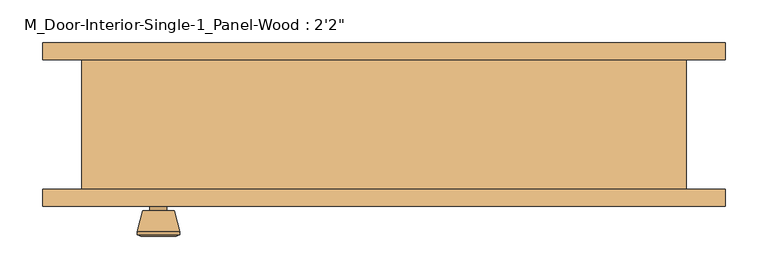
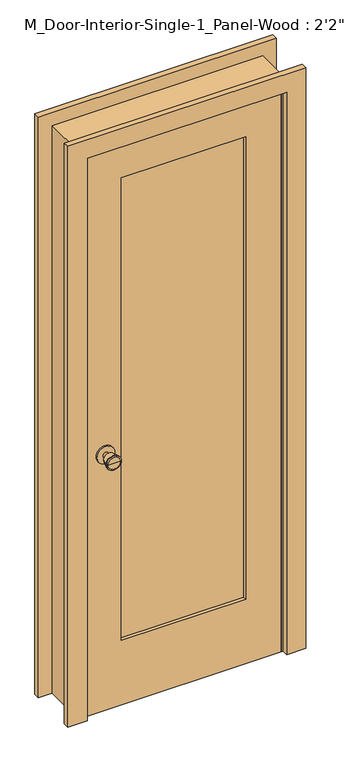
"""IFC4 building model written with IfcOpenShell, lengths in millimetres: door geometry."""

from ifc_helpers import new_model, si_unit, point, frame, frame_2d, origin, place, context, project, spatial, polyline, circle_curve, trimmed, segment, composite_curve, outline, extrude, faceted_brep, source, transform, mapped, element, save
from ifc_brep_helpers import plane_surface, cylinder_surface, revolved_surface, advanced_brep


def door_acb0f330(model_context):
    return source(origin(), model_context, "Body", "SolidModel", [
        advanced_brep(
        [(-265.2, -32.025, 914.4), (-275.2, -32.025, 914.4), (-255.2, -32.025, 914.4), (-244.7241324, 16.975, 914.4), (-285.6758676, 16.975, 914.4), (-265.2, 16.975, 914.4), (-240.2, 15.1471319, 914.4), (-290.2, 15.1471319, 914.4), (-240.2, 11.6834537, 914.4), (-290.2, 11.6834537, 914.4), (-246.563764, -13.025, 914.4), (-283.836236, -13.025, 914.4), (-255.2, -13.025, 914.4), (-275.2, -13.025, 914.4)],
        [
            (0, 1),
            (1, 2, circle_curve(frame((-265.2, -32.025, 914.4), z_axis=(0.0, -1.0, 0.0), x_axis=(-1.0, 0.0, 0.0)), 10.0)),
            (2, 0),
            (2, 1, circle_curve(frame((-265.2, -32.025, 914.4), z_axis=(0.0, -1.0, 0.0), x_axis=(-1.0, 0.0, 0.0)), 10.0)),
            (3, 4, circle_curve(frame((-265.2, 16.975, 914.4), z_axis=(0.0, 1.0, 0.0), x_axis=(-1.0, 0.0, 0.0)), 20.4758676)),
            (4, 5),
            (5, 3),
            (4, 3, circle_curve(frame((-265.2, 16.975, 914.4), z_axis=(0.0, 1.0, 0.0), x_axis=(-1.0, 0.0, 0.0)), 20.4758676)),
            (6, 7, circle_curve(frame((-265.2, 15.1471319, 914.4), z_axis=(0.0, 1.0, 0.0), x_axis=(-1.0, 0.0, 0.0)), 25.0)),
            (7, 4),
            (3, 6),
            (7, 6, circle_curve(frame((-265.2, 15.1471319, 914.4), z_axis=(0.0, 1.0, 0.0), x_axis=(-1.0, 0.0, 0.0)), 25.0)),
            (8, 9, circle_curve(frame((-265.2, 11.6834537, 914.4), z_axis=(0.0, 1.0, 0.0), x_axis=(-1.0, 0.0, 0.0)), 25.0)),
            (9, 7),
            (6, 8),
            (9, 8, circle_curve(frame((-265.2, 11.6834537, 914.4), z_axis=(0.0, 1.0, 0.0), x_axis=(-1.0, 0.0, 0.0)), 25.0)),
            (10, 11, circle_curve(frame((-265.2, -13.025, 914.4), z_axis=(0.0, 1.0, 0.0), x_axis=(-1.0, 0.0, 0.0)), 18.636236)),
            (11, 9),
            (8, 10),
            (11, 10, circle_curve(frame((-265.2, -13.025, 914.4), z_axis=(0.0, 1.0, 0.0), x_axis=(-1.0, 0.0, 0.0)), 18.636236)),
            (12, 13, circle_curve(frame((-265.2, -13.025, 914.4), z_axis=(0.0, 1.0, 0.0), x_axis=(-1.0, 0.0, 0.0)), 10.0)),
            (13, 11),
            (10, 12),
            (13, 12, circle_curve(frame((-265.2, -13.025, 914.4), z_axis=(0.0, 1.0, 0.0), x_axis=(-1.0, 0.0, 0.0)), 10.0)),
            (1, 13),
            (12, 2),
        ],
        [
            plane_surface(frame((-265.2, -32.025, 914.4), z_axis=(0.0, -1.0, 0.0), x_axis=(-1.0, 0.0, 0.0))),
            plane_surface(frame((-265.2, 16.975, 914.4), z_axis=(0.0, 1.0, 0.0), x_axis=(-1.0, 0.0, 0.0))),
            revolved_surface(polyline([(-285.6758676, 16.975, 914.4), (-290.2, 15.1471319, 914.4)]), (-265.2, -32.025, 914.4), (0.0, -1.0, 0.0)),
            cylinder_surface(frame((-265.2, -32.025, 914.4), z_axis=(0.0, -1.0, 0.0), x_axis=(-1.0, 0.0, 0.0)), 25.0),
            revolved_surface(polyline([(-290.2, 11.6834537, 914.4), (-283.836236, -13.025, 914.4)]), (-265.2, -32.025, 914.4), (0.0, -1.0, 0.0)),
            plane_surface(frame((-265.2, -13.025, 914.4), z_axis=(0.0, -1.0, 0.0), x_axis=(-1.0, 0.0, 0.0))),
            cylinder_surface(frame((-265.2, -32.025, 914.4), z_axis=(0.0, -1.0, 0.0), x_axis=(-1.0, 0.0, 0.0)), 10.0),
        ],
        [
            (0, [[1, 2, 3]]),
            (0, [[-3, 4, -1]]),
            (1, [[5, 6, 7]]),
            (1, [[8, -7, -6]]),
            (2, [[9, 10, -5, 11]]),
            (2, [[12, -11, -8, -10]]),
            (3, [[13, 14, -9, 15]]),
            (3, [[16, -15, -12, -14]]),
            (4, [[17, 18, -13, 19]]),
            (4, [[20, -19, -16, -18]]),
            (5, [[21, 22, -17, 23]]),
            (5, [[24, -23, -20, -22]]),
            (6, [[-2, 25, -21, 26]]),
            (6, [[-4, -26, -24, -25]]),
        ],
    ),
        extrude(outline(composite_curve([segment(trimmed(circle_curve(frame_2d((914.4, -265.2)), 30.0), [point((914.4, -295.2))], [point((914.4, -235.2))], False, "CARTESIAN"), True, "CONTINUOUS"), segment(trimmed(circle_curve(frame_2d((914.4, -265.2)), 30.0), [point((914.4, -235.2))], [point((914.4, -295.2))], False, "CARTESIAN"), True, "CONTINUOUS")], self_intersect=False)), frame((0.0, -38.025, 0.0), z_axis=(0.0, 1.0, 0.0), x_axis=(0.0, 0.0, 1.0)), (0.0, 0.0, 1.0), 6.0),
        advanced_brep(
        [(-265.2, -79.025, 914.4), (-255.2, -79.025, 914.4), (-275.2, -79.025, 914.4), (-244.7241324, -128.025, 914.4), (-265.2, -128.025, 914.4), (-285.6758676, -128.025, 914.4), (-240.2, -126.1971319, 914.4), (-290.2, -126.1971319, 914.4), (-240.2, -122.7334537, 914.4), (-290.2, -122.7334537, 914.4), (-246.563764, -98.025, 914.4), (-283.836236, -98.025, 914.4), (-255.2, -98.025, 914.4), (-275.2, -98.025, 914.4)],
        [
            (0, 1),
            (1, 2, circle_curve(frame((-265.2, -79.025, 914.4), z_axis=(0.0, 1.0, 0.0), x_axis=(-1.0, 0.0, 0.0)), 10.0)),
            (2, 0),
            (2, 1, circle_curve(frame((-265.2, -79.025, 914.4), z_axis=(0.0, 1.0, 0.0), x_axis=(-1.0, 0.0, 0.0)), 10.0)),
            (3, 4),
            (4, 5),
            (5, 3, circle_curve(frame((-265.2, -128.025, 914.4), z_axis=(0.0, -1.0, 0.0), x_axis=(-1.0, 0.0, 0.0)), 20.4758676)),
            (3, 5, circle_curve(frame((-265.2, -128.025, 914.4), z_axis=(0.0, -1.0, 0.0), x_axis=(-1.0, 0.0, 0.0)), 20.4758676)),
            (6, 3),
            (5, 7),
            (7, 6, circle_curve(frame((-265.2, -126.1971319, 914.4), z_axis=(0.0, -1.0, 0.0), x_axis=(-1.0, 0.0, 0.0)), 25.0)),
            (6, 7, circle_curve(frame((-265.2, -126.1971319, 914.4), z_axis=(0.0, -1.0, 0.0), x_axis=(-1.0, 0.0, 0.0)), 25.0)),
            (8, 6),
            (7, 9),
            (9, 8, circle_curve(frame((-265.2, -122.7334537, 914.4), z_axis=(0.0, -1.0, 0.0), x_axis=(-1.0, 0.0, 0.0)), 25.0)),
            (8, 9, circle_curve(frame((-265.2, -122.7334537, 914.4), z_axis=(0.0, -1.0, 0.0), x_axis=(-1.0, 0.0, 0.0)), 25.0)),
            (10, 8),
            (9, 11),
            (11, 10, circle_curve(frame((-265.2, -98.025, 914.4), z_axis=(0.0, -1.0, 0.0), x_axis=(-1.0, 0.0, 0.0)), 18.636236)),
            (10, 11, circle_curve(frame((-265.2, -98.025, 914.4), z_axis=(0.0, -1.0, 0.0), x_axis=(-1.0, 0.0, 0.0)), 18.636236)),
            (12, 10),
            (11, 13),
            (13, 12, circle_curve(frame((-265.2, -98.025, 914.4), z_axis=(0.0, -1.0, 0.0), x_axis=(-1.0, 0.0, 0.0)), 10.0)),
            (12, 13, circle_curve(frame((-265.2, -98.025, 914.4), z_axis=(0.0, -1.0, 0.0), x_axis=(-1.0, 0.0, 0.0)), 10.0)),
            (1, 12),
            (13, 2),
        ],
        [
            plane_surface(frame((-265.2, -79.025, 914.4), z_axis=(0.0, 1.0, 0.0), x_axis=(-1.0, 0.0, 0.0))),
            plane_surface(frame((-265.2, -128.025, 914.4), z_axis=(0.0, -1.0, 0.0), x_axis=(-1.0, 0.0, 0.0))),
            revolved_surface(polyline([(-285.6758676, -128.025, 914.4), (-290.2, -126.1971319, 914.4)]), (-265.2, -79.025, 914.4), (0.0, 1.0, 0.0)),
            cylinder_surface(frame((-265.2, -79.025, 914.4), z_axis=(0.0, 1.0, 0.0), x_axis=(-1.0, 0.0, 0.0)), 25.0),
            revolved_surface(polyline([(-290.2, -122.7334537, 914.4), (-283.836236, -98.025, 914.4)]), (-265.2, -79.025, 914.4), (0.0, 1.0, 0.0)),
            plane_surface(frame((-265.2, -98.025, 914.4), z_axis=(0.0, 1.0, 0.0), x_axis=(-1.0, 0.0, 0.0))),
            cylinder_surface(frame((-265.2, -79.025, 914.4), z_axis=(0.0, 1.0, 0.0), x_axis=(-1.0, 0.0, 0.0)), 10.0),
        ],
        [
            (0, [[1, 2, 3]]),
            (0, [[-3, 4, -1]]),
            (1, [[5, 6, 7]]),
            (1, [[-6, -5, 8]]),
            (2, [[9, -7, 10, 11]]),
            (2, [[-10, -8, -9, 12]]),
            (3, [[13, -11, 14, 15]]),
            (3, [[-14, -12, -13, 16]]),
            (4, [[17, -15, 18, 19]]),
            (4, [[-18, -16, -17, 20]]),
            (5, [[21, -19, 22, 23]]),
            (5, [[-22, -20, -21, 24]]),
            (6, [[25, -23, 26, -2]]),
            (6, [[-26, -24, -25, -4]]),
        ],
    ),
        extrude(outline(composite_curve([segment(trimmed(circle_curve(frame_2d((914.4, -265.2)), 30.0), [point((914.4, -295.2))], [point((914.4, -235.2))], False, "CARTESIAN"), True, "CONTINUOUS"), segment(trimmed(circle_curve(frame_2d((914.4, -265.2)), 30.0), [point((914.4, -235.2))], [point((914.4, -295.2))], False, "CARTESIAN"), True, "CONTINUOUS")], self_intersect=False)), frame((0.0, -79.025, 0.0), z_axis=(0.0, 1.0, 0.0), x_axis=(0.0, 0.0, 1.0)), (0.0, 0.0, 1.0), 6.0),
        faceted_brep([(355.2, -73.025, 0.0), (330.2, -73.025, 0.0), (330.2, -38.025, 0.0), (317.5, -38.025, 0.0), (317.5, -3.1, 0.0), (330.2, -3.1, 0.0), (330.2, 79.375, 0.0), (355.2, 79.375, 0.0), (355.2, 79.375, 2025.0), (355.2, -73.025, 2025.0), (330.2, 79.375, 2000.0), (-330.2, 79.375, 2000.0), (-330.2, 79.375, 0.0), (-355.2, 79.375, 0.0), (-355.2, 79.375, 2025.0), (330.2, -3.1, 2000.0), (317.5, -3.1, 1987.3), (-317.5, -3.1, 1987.3), (-317.5, -3.1, 0.0), (-330.2, -3.1, 0.0), (-330.2, -3.1, 2000.0), (317.5, -38.025, 1987.3), (330.2, -38.025, 2000.0), (-330.2, -38.025, 2000.0), (-330.2, -38.025, 0.0), (-317.5, -38.025, 0.0), (-317.5, -38.025, 1987.3), (330.2, -73.025, 2000.0), (-355.2, -73.025, 2025.0), (-355.2, -73.025, 0.0), (-330.2, -73.025, 0.0), (-330.2, -73.025, 2000.0)], [[[0, 1, 2, 3, 4, 5, 6, 7]], [[7, 8, 9, 0]], [[6, 10, 11, 12, 13, 14, 8, 7]], [[5, 15, 10, 6]], [[4, 16, 17, 18, 19, 20, 15, 5]], [[3, 21, 16, 4]], [[2, 22, 23, 24, 25, 26, 21, 3]], [[1, 27, 22, 2]], [[0, 9, 28, 29, 30, 31, 27, 1]], [[8, 14, 28, 9]], [[15, 20, 11, 10]], [[21, 26, 17, 16]], [[27, 31, 23, 22]], [[29, 13, 12, 19, 18, 25, 24, 30]], [[14, 13, 29, 28]], [[20, 19, 12, 11]], [[26, 25, 18, 17]], [[31, 30, 24, 23]]]),
        extrude(outline(polyline([(2000.0, -330.2), (0.0, -330.2), (0.0, 330.2), (2000.0, 330.2), (2000.0, -330.2)]), holes=[polyline([(1880.0, -210.2), (1880.0, 210.2), (230.0, 210.2), (230.0, -210.2), (1880.0, -210.2)])]), frame((0.0, -73.025, 0.0), z_axis=(0.0, 1.0, 0.0), x_axis=(0.0, 0.0, 1.0)), (0.0, 0.0, 1.0), 35.0),
        extrude(outline(polyline([(210.2, -49.6916667), (210.2, -61.3583333), (-210.2, -61.3583333), (-210.2, -49.6916667), (210.2, -49.6916667)])), frame((0.0, 0.0, 230.0), z_axis=(0.0, 0.0, 1.0), x_axis=(1.0, 0.0, 0.0)), (0.0, 0.0, 1.0), 1650.0),
        extrude(outline(polyline([(0.0, 401.55), (2071.35, 401.55), (2071.35, -401.55), (0.0, -401.55), (0.0, -336.55), (2006.35, -336.55), (2006.35, 336.55), (0.0, 336.55), (0.0, 401.55)])), frame((0.0, -93.025, 0.0), z_axis=(0.0, 1.0, 0.0), x_axis=(0.0, 0.0, 1.0)), (0.0, 0.0, 1.0), 20.0),
        extrude(outline(polyline([(0.0, 401.55), (2071.35, 401.55), (2071.35, -401.55), (0.0, -401.55), (0.0, -336.55), (2006.35, -336.55), (2006.35, 336.55), (0.0, 336.55), (0.0, 401.55)])), frame((0.0, 79.375, 0.0), z_axis=(0.0, 1.0, 0.0), x_axis=(0.0, 0.0, 1.0)), (0.0, 0.0, 1.0), 20.0),
    ])


if __name__ == "__main__":
    model = new_model("IFC4")
    model_context = context("Model", 3, world=origin())
    ifc_project = project(units=[si_unit("LENGTHUNIT", "METRE", prefix="MILLI")], contexts=[model_context])
    site = spatial("IfcSite", under=ifc_project)
    building = spatial("IfcBuilding", under=site)
    placement = place(None, origin())
    door_shape = door_acb0f330(model_context)
    element("IfcDoor", 1, ObjectType="M_Door-Interior-Single-1_Panel-Wood : 2'2\"", at=placement, inside=building, context=model_context, shape_type="MappedRepresentation", body=[
        mapped(door_shape, transform((0.0, 0.0, 0.0), x_axis=(1.0, 0.0, 0.0), y_axis=(0.0, 1.0, 0.0), z_axis=(0.0, 0.0, 1.0))),
    ])
    save(model, "model.ifc")

# Revit data of these elements
# Type "M_Door-Interior-Single-1_Panel-Wood : 2'2\""
#   Type Mark = "17"
#   Assembly Code = "C1020300"
#   Analytic Construction = "Wooden"
#   Top Rail = 0' - 4.72441"
#   Thickness = 0' - 1.37795"
#   Thermal Resistance (R) = 2.5876 (h·ft²·°F)/BTU
#   Swing Angle [instance default] = 90.00°
#   Stiles = 0' - 4.72441"
#   Rough Width = 2' - 3.9685"
#   Rough Height = 6' - 7.72441"
#   Height = 6' - 6.74016"
#   Width = 2' - 2"
#   Heat Transfer Coefficient (U) = 0.3865 BTU/(h·ft²·°F)
#   Bottom Rail = 0' - 9.05512"
#   Trim Material = Cherry
#   Panel Material = Cherry
#   Frame Material = Cherry
#   Door Handle Material = Aluminum
#   Visual Light Transmittance = 0
#   Solar Heat Gain Coefficient = 0
#   Wall Closure = (empty or 0)
#   Function = (empty or 0)
# Element 1 (IfcDoor, "M_Door-Interior-Single-1_Panel-Wood : 2'2\"")
#   Materials on its faces: "Cherry", "Aluminum"
# Materials
#   "Cherry": class "Wood", colour RGB 226 177 128, transparency 0, Description = "Prunus Serotina", Cost = 0
#   "Aluminum": class "Metal", colour RGB 247 247 247, transparency 0, Description = "Aluminum 6061", Cost = 0
